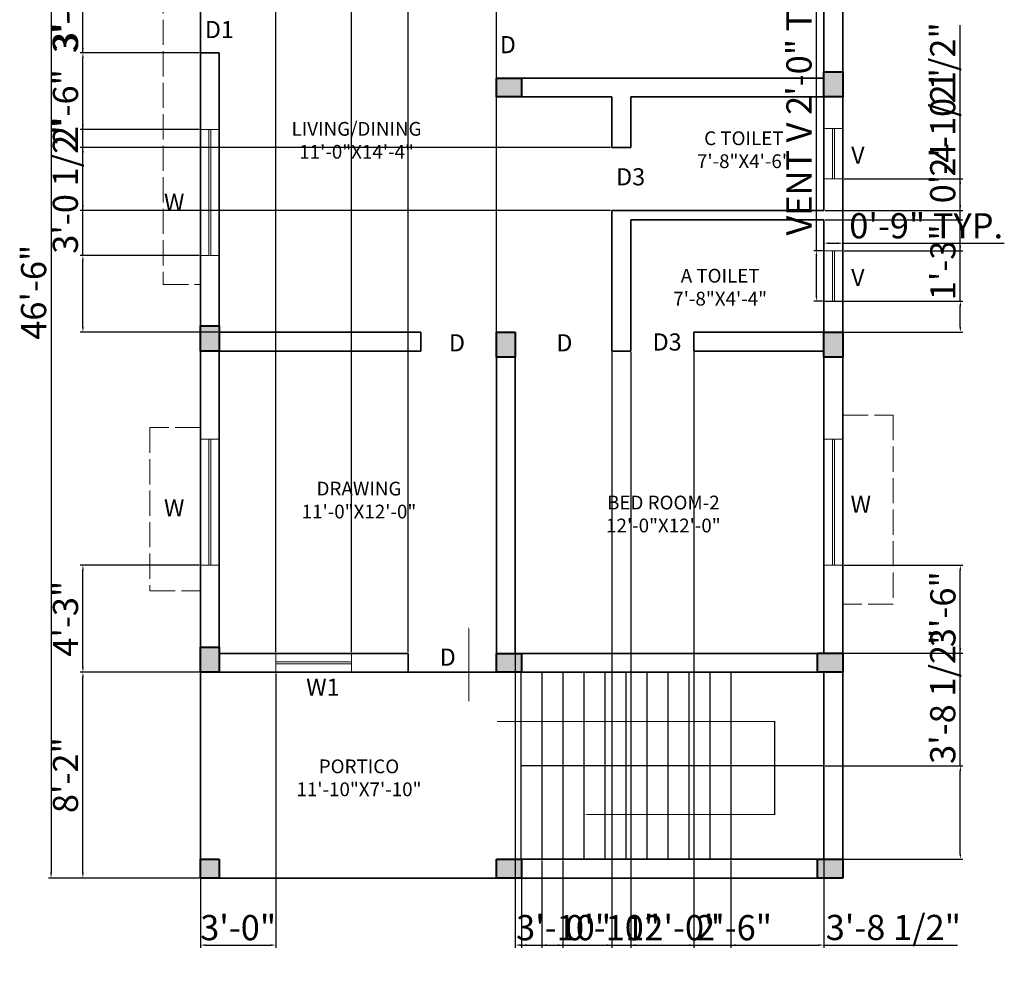
# Model space of a CAD drawing. Units: inches. Extents: x 27449 to 27965, y 46348 to 47103.
# Tile 1 of 2: x 27449 to 27918, y 46348 to 46800. Entities that reach past the tile are written whole.
import ezdxf

# ---------------------------------------------------------------- set-up
doc = ezdxf.new("R2010")
doc.units = ezdxf.units.IN
doc.linetypes.add('ACAD_ISO02W100', pattern=[15, 12, -3])
for name, color, linetype, lineweight in [('A-ANNO-DIMS', 2, 'Continuous', 18), ('A-ANNO-SYMB', 7, 'Continuous', 18), ('A-ANNO-TEXT', 7, 'Continuous', 18), ('A-AREA-IDEN', 7, 'Continuous', 20), ('A-COLS', 7, 'Continuous', 40), ('A-COLS-PATT', 252, 'Continuous', 13), ('A-FLOR-STRS', 7, 'Continuous', 25), ('A-GLAZ', 4, 'Continuous', 20), ('A-GLAZ-OVHD', 8, 'ACAD_ISO02W100', 13), ('A-WALL', 7, 'Continuous', 35)]:
    doc.layers.add(name, color=color, linetype=linetype, lineweight=lineweight)
doc.styles.get("Standard").update_dxf_attribs({"font": 'arial.ttf'})
doc.dimstyles.new('ISO-25', dxfattribs={"dimtxt": 12, "dimasz": 2.5, "dimexe": 1.25, "dimexo": 0.625, "dimtad": 1, "dimlunit": 3, "dimtxsty": 'Standard', "dimcen": 2.5, "dimadec": 0, "dimazin": 0, "dimtfac": 1, "dimtmove": 0, "dimatfit": 3, "dimfxl": 1, "dimarcsym": 0})

# ---------------------------------------------------------------- blocks, each defined once
blk = doc.blocks.new('*D1')
at = {"layer": 'A-ANNO-DIMS', "color": 0, "lineweight": -2, "transparency": 16777216}
for p, q in [((27534.79, 46948.86), (27463.05, 46948.86)), ((27464.3, 46946.36), (27464.3, 46393.36)), ((27534.79, 46390.86), (27463.05, 46390.86))]:
    blk.add_line(p, q, dxfattribs=at)
at = {"layer": 'A-ANNO-DIMS', "color": 0, "transparency": 16777216}
for points in [[(27463.88, 46946.36), (27464.71, 46946.36), (27464.3, 46948.86)], [(27463.88, 46393.36), (27464.71, 46393.36), (27464.3, 46390.86)]]:
    blk.add_solid(points, dxfattribs=at)
at = {"layer": 'Defpoints', "color": 0, "transparency": 16777216}
for p in [(27535.42, 46948.86), (27464.3, 46390.86), (27535.42, 46390.86)]:
    blk.add_point(p, dxfattribs=at)
at = {"layer": 'A-ANNO-DIMS', "color": 0, "transparency": 16777216, "insert": (27457.54, 46669.86), "char_height": 12, "attachment_point": 5, "rotation": 90}
blk.add_mtext('46\'-6"', dxfattribs=at)
blk = doc.blocks.new('WIN-W-60IN')
for p, q in [((0, 60), (9, 60)), ((0, 0), (0, 60)), ((4, 0), (4, 60)), ((5, 0), (5, 60)), ((9, 60), (9, 0)), ((9, 0), (0, 0))]:
    blk.add_line(p, q)
blk = doc.blocks.new('VENT-V-24IN')
for p, q in [((0, 0), (0, 24)), ((0, 24), (9, 24)), ((4, 24), (4, 0)), ((5, 24), (5, 0)), ((9, 24), (9, 0)), ((0, 0), (9, 0))]:
    blk.add_line(p, q)
blk = doc.blocks.new('COL-9X12IN')
h = blk.add_hatch(color=256)
h.dxf.hatch_style = 1
h.paths.add_polyline_path([(9, 12), (0, 12), (0, 0), (9, 0)])
for p, q in [((0, 12), (9, 12)), ((0, 0), (0, 12)), ((9, 12), (9, 0)), ((9, 0), (0, 0))]:
    blk.add_line(p, q)
blk = doc.blocks.new('ENTRY-ARROW')
blk.add_lwpolyline([(0, 0, 0.5, 0.5, 0), (0, 22.23, 5, 0, 0), (0, 35.55, 0, 0, 0)], format="xyseb")
blk = doc.blocks.new('*D11')
at = {"layer": 'A-ANNO-DIMS', "color": 0, "lineweight": -2, "transparency": 16777216}
for p, q in [((27828.82, 46689.61), (27828.82, 46832.34)), ((27831.79, 46689.61), (27827.57, 46689.61)), ((27828.82, 46668.11), (27828.82, 46687.11)), ((27831.79, 46665.61), (27827.57, 46665.61))]:
    blk.add_line(p, q, dxfattribs=at)
at = {"layer": 'A-ANNO-DIMS', "color": 0, "transparency": 16777216}
for points in [[(27828.4, 46687.11), (27829.24, 46687.11), (27828.82, 46689.61)], [(27828.4, 46668.11), (27829.24, 46668.11), (27828.82, 46665.61)]]:
    blk.add_solid(points, dxfattribs=at)
at = {"layer": 'Defpoints', "color": 0, "transparency": 16777216}
for p in [(27828.82, 46689.61), (27832.42, 46689.61), (27832.42, 46665.61)]:
    blk.add_point(p, dxfattribs=at)
at = {"layer": 'A-ANNO-DIMS', "color": 0, "transparency": 16777216, "insert": (27822.07, 46762.22), "char_height": 12, "attachment_point": 5, "rotation": 90}
blk.add_mtext('VENT V 2\'-0" TYP.', dxfattribs=at)
blk = doc.blocks.new('*D12')
at = {"layer": 'A-ANNO-DIMS', "color": 0, "lineweight": -2, "transparency": 16777216}
for p, q in [((27832.42, 46690.24), (27832.42, 46694.46)), ((27841.42, 46690.24), (27841.42, 46694.46)), ((27834.92, 46693.21), (27838.92, 46693.21)), ((27841.42, 46693.21), (27918.32, 46693.21))]:
    blk.add_line(p, q, dxfattribs=at)
at = {"layer": 'A-ANNO-DIMS', "color": 0, "transparency": 16777216}
for points in [[(27834.92, 46693.63), (27834.92, 46692.8), (27832.42, 46693.21)], [(27838.92, 46693.63), (27838.92, 46692.8), (27841.42, 46693.21)]]:
    blk.add_solid(points, dxfattribs=at)
at = {"layer": 'Defpoints', "color": 0, "transparency": 16777216}
for p in [(27832.42, 46689.61), (27841.42, 46693.21), (27841.42, 46689.61)]:
    blk.add_point(p, dxfattribs=at)
at = {"layer": 'A-ANNO-DIMS', "color": 0, "transparency": 16777216, "insert": (27881.12, 46699.96), "char_height": 12, "attachment_point": 5}
blk.add_mtext('0\'-9" TYP.', dxfattribs=at)
blk = doc.blocks.new('*D13')
at = {"layer": 'A-ANNO-DIMS', "color": 0, "lineweight": -2, "transparency": 16777216}
for p, q in [((27534.79, 46488.86), (27478.22, 46488.86)), ((27479.47, 46393.36), (27479.47, 46486.36)), ((27534.79, 46390.86), (27478.22, 46390.86))]:
    blk.add_line(p, q, dxfattribs=at)
at = {"layer": 'A-ANNO-DIMS', "color": 0, "transparency": 16777216}
for points in [[(27479.05, 46486.36), (27479.89, 46486.36), (27479.47, 46488.86)], [(27479.05, 46393.36), (27479.89, 46393.36), (27479.47, 46390.86)]]:
    blk.add_solid(points, dxfattribs=at)
at = {"layer": 'Defpoints', "color": 0, "transparency": 16777216}
for p in [(27479.47, 46488.86), (27535.42, 46488.86), (27535.42, 46390.86)]:
    blk.add_point(p, dxfattribs=at)
at = {"layer": 'A-ANNO-DIMS', "color": 0, "transparency": 16777216, "insert": (27472.72, 46439.86), "char_height": 12, "attachment_point": 5, "rotation": 90}
blk.add_mtext('8\'-2"', dxfattribs=at)
blk = doc.blocks.new('*D14')
at = {"layer": 'A-ANNO-DIMS', "color": 0, "lineweight": -2, "transparency": 16777216}
for p, q in [((27534.79, 46539.86), (27478.22, 46539.86)), ((27479.47, 46491.36), (27479.47, 46537.36)), ((27534.79, 46488.86), (27478.22, 46488.86))]:
    blk.add_line(p, q, dxfattribs=at)
at = {"layer": 'A-ANNO-DIMS', "color": 0, "transparency": 16777216}
for points in [[(27479.05, 46537.36), (27479.89, 46537.36), (27479.47, 46539.86)], [(27479.05, 46491.36), (27479.89, 46491.36), (27479.47, 46488.86)]]:
    blk.add_solid(points, dxfattribs=at)
at = {"layer": 'Defpoints', "color": 0, "transparency": 16777216}
for p in [(27479.47, 46539.86), (27535.42, 46539.86), (27535.42, 46488.86)]:
    blk.add_point(p, dxfattribs=at)
at = {"layer": 'A-ANNO-DIMS', "color": 0, "transparency": 16777216, "insert": (27472.71, 46514.36), "char_height": 12, "attachment_point": 5, "rotation": 90}
blk.add_mtext('4\'-3"', dxfattribs=at)
blk = doc.blocks.new('*D15')
at = {"layer": 'A-ANNO-DIMS', "color": 0, "lineweight": -2, "transparency": 16777216}
for p, q in [((27479.47, 46687.36), (27479.47, 46750.97)), ((27534.79, 46687.36), (27478.22, 46687.36)), ((27479.47, 46653.36), (27479.47, 46684.86)), ((27543.79, 46650.86), (27478.22, 46650.86))]:
    blk.add_line(p, q, dxfattribs=at)
at = {"layer": 'A-ANNO-DIMS', "color": 0, "transparency": 16777216}
for points in [[(27479.05, 46684.86), (27479.89, 46684.86), (27479.47, 46687.36)], [(27479.05, 46653.36), (27479.89, 46653.36), (27479.47, 46650.86)]]:
    blk.add_solid(points, dxfattribs=at)
at = {"layer": 'Defpoints', "color": 0, "transparency": 16777216}
for p in [(27479.47, 46687.36), (27535.42, 46687.36), (27544.42, 46650.86)]:
    blk.add_point(p, dxfattribs=at)
at = {"layer": 'A-ANNO-DIMS', "color": 0, "transparency": 16777216, "insert": (27472.64, 46720.41), "char_height": 12, "attachment_point": 5, "rotation": 90}
blk.add_mtext('3\'-0 1/2"', dxfattribs=at)
blk = doc.blocks.new('*D16')
at = {"layer": 'A-ANNO-DIMS', "color": 0, "lineweight": -2, "transparency": 16777216}
for p, q in [((27479.47, 46783.86), (27479.47, 46847.47)), ((27534.79, 46783.86), (27478.22, 46783.86)), ((27479.47, 46749.86), (27479.47, 46781.36)), ((27534.79, 46747.36), (27478.22, 46747.36))]:
    blk.add_line(p, q, dxfattribs=at)
at = {"layer": 'A-ANNO-DIMS', "color": 0, "transparency": 16777216}
for points in [[(27479.05, 46781.36), (27479.89, 46781.36), (27479.47, 46783.86)], [(27479.05, 46749.86), (27479.89, 46749.86), (27479.47, 46747.36)]]:
    blk.add_solid(points, dxfattribs=at)
at = {"layer": 'Defpoints', "color": 0, "transparency": 16777216}
for p in [(27479.47, 46783.86), (27535.42, 46783.86), (27535.42, 46747.36)]:
    blk.add_point(p, dxfattribs=at)
at = {"layer": 'A-ANNO-DIMS', "color": 0, "transparency": 16777216, "insert": (27472.64, 46816.91), "char_height": 12, "attachment_point": 5, "rotation": 90}
blk.add_mtext('3\'-0 1/2"', dxfattribs=at)
blk = doc.blocks.new('*D17')
at = {"layer": 'A-ANNO-DIMS', "color": 0, "lineweight": -2, "transparency": 16777216}
for p, q in [((27534.79, 46819.86), (27478.22, 46819.86)), ((27479.47, 46786.36), (27479.47, 46817.36)), ((27534.79, 46783.86), (27478.22, 46783.86))]:
    blk.add_line(p, q, dxfattribs=at)
at = {"layer": 'A-ANNO-DIMS', "color": 0, "transparency": 16777216}
for points in [[(27479.05, 46817.36), (27479.89, 46817.36), (27479.47, 46819.86)], [(27479.05, 46786.36), (27479.89, 46786.36), (27479.47, 46783.86)]]:
    blk.add_solid(points, dxfattribs=at)
at = {"layer": 'Defpoints', "color": 0, "transparency": 16777216}
for p in [(27479.47, 46819.86), (27535.42, 46819.86), (27535.42, 46783.86)]:
    blk.add_point(p, dxfattribs=at)
at = {"layer": 'A-ANNO-DIMS', "color": 0, "transparency": 16777216, "insert": (27472.71, 46801.86), "char_height": 12, "attachment_point": 5, "rotation": 90}
blk.add_mtext('3\'-0"', dxfattribs=at)
blk = doc.blocks.new('*D20')
at = {"layer": 'A-ANNO-DIMS', "color": 0, "lineweight": -2, "transparency": 16777216}
for p, q in [((27571.42, 46498.49), (27571.42, 47006.06)), ((27573.92, 47004.81), (27604.92, 47004.81)), ((27607.42, 46498.49), (27607.42, 47006.06))]:
    blk.add_line(p, q, dxfattribs=at)
at = {"layer": 'A-ANNO-DIMS', "color": 0, "transparency": 16777216}
for points in [[(27573.92, 47005.23), (27573.92, 47004.4), (27571.42, 47004.81)], [(27604.92, 47005.23), (27604.92, 47004.4), (27607.42, 47004.81)]]:
    blk.add_solid(points, dxfattribs=at)
at = {"layer": 'Defpoints', "color": 0, "transparency": 16777216}
for p in [(27607.42, 47004.81), (27571.42, 46497.86), (27607.42, 46497.86)]:
    blk.add_point(p, dxfattribs=at)
at = {"layer": 'A-ANNO-DIMS', "color": 0, "transparency": 16777216, "insert": (27589.42, 47011.57), "char_height": 12, "attachment_point": 5}
blk.add_mtext('3\'-0"', dxfattribs=at)
blk = doc.blocks.new('*D21')
at = {"layer": 'A-ANNO-DIMS', "color": 0, "lineweight": -2, "transparency": 16777216}
for p, q in [((27535.42, 46488.24), (27535.42, 46357.66)), ((27571.42, 46488.24), (27571.42, 46357.66)), ((27537.92, 46358.91), (27568.92, 46358.91))]:
    blk.add_line(p, q, dxfattribs=at)
at = {"layer": 'A-ANNO-DIMS', "color": 0, "transparency": 16777216}
for points in [[(27537.92, 46359.33), (27537.92, 46358.5), (27535.42, 46358.91)], [(27568.92, 46359.33), (27568.92, 46358.5), (27571.42, 46358.91)]]:
    blk.add_solid(points, dxfattribs=at)
at = {"layer": 'Defpoints', "color": 0, "transparency": 16777216}
for p in [(27535.42, 46488.86), (27571.42, 46488.86), (27571.42, 46358.91)]:
    blk.add_point(p, dxfattribs=at)
at = {"layer": 'A-ANNO-DIMS', "color": 0, "transparency": 16777216, "insert": (27553.42, 46365.67), "char_height": 12, "attachment_point": 5}
blk.add_mtext('3\'-0"', dxfattribs=at)
blk = doc.blocks.new('*D22')
at = {"layer": 'A-ANNO-DIMS', "color": 0, "lineweight": -2, "transparency": 16777216}
for p, q in [((27634.42, 46498.49), (27634.42, 47006.06)), ((27636.92, 47004.81), (27673.92, 47004.81)), ((27676.42, 46498.49), (27676.42, 47006.06))]:
    blk.add_line(p, q, dxfattribs=at)
at = {"layer": 'A-ANNO-DIMS', "color": 0, "transparency": 16777216}
for points in [[(27636.92, 47005.23), (27636.92, 47004.4), (27634.42, 47004.81)], [(27673.92, 47005.23), (27673.92, 47004.4), (27676.42, 47004.81)]]:
    blk.add_solid(points, dxfattribs=at)
at = {"layer": 'Defpoints', "color": 0, "transparency": 16777216}
for p in [(27676.42, 47004.81), (27634.42, 46497.86), (27676.42, 46497.86)]:
    blk.add_point(p, dxfattribs=at)
at = {"layer": 'A-ANNO-DIMS', "color": 0, "transparency": 16777216, "insert": (27655.42, 47011.57), "char_height": 12, "attachment_point": 5}
blk.add_mtext('3\'-6"', dxfattribs=at)
blk = doc.blocks.new('*D23')
at = {"layer": 'A-ANNO-DIMS', "color": 0, "lineweight": -2, "transparency": 16777216}
for p, q in [((27688.42, 46399.24), (27688.42, 46357.66)), ((27832.42, 46399.24), (27832.42, 46357.66)), ((27690.92, 46358.91), (27829.92, 46358.91))]:
    blk.add_line(p, q, dxfattribs=at)
at = {"layer": 'A-ANNO-DIMS', "color": 0, "transparency": 16777216}
for points in [[(27690.92, 46359.33), (27690.92, 46358.5), (27688.42, 46358.91)], [(27829.92, 46359.33), (27829.92, 46358.5), (27832.42, 46358.91)]]:
    blk.add_solid(points, dxfattribs=at)
at = {"layer": 'Defpoints', "color": 0, "transparency": 16777216}
for p in [(27688.42, 46399.86), (27832.42, 46399.86), (27832.42, 46358.91)]:
    blk.add_point(p, dxfattribs=at)
at = {"layer": 'A-ANNO-DIMS', "color": 0, "transparency": 16777216, "insert": (27760.42, 46365.66), "char_height": 12, "attachment_point": 5}
blk.add_mtext('12\'-0"', dxfattribs=at)
blk = doc.blocks.new('*D24')
at = {"layer": 'A-ANNO-DIMS', "color": 0, "lineweight": -2, "transparency": 16777216}
for p, q in [((27788.02, 46399.24), (27788.02, 46357.66)), ((27832.42, 46399.24), (27832.42, 46357.66)), ((27790.52, 46358.91), (27829.92, 46358.91)), ((27832.42, 46358.91), (27896.02, 46358.91))]:
    blk.add_line(p, q, dxfattribs=at)
at = {"layer": 'A-ANNO-DIMS', "color": 0, "transparency": 16777216}
for points in [[(27790.52, 46359.33), (27790.52, 46358.5), (27788.02, 46358.91)], [(27829.92, 46359.33), (27829.92, 46358.5), (27832.42, 46358.91)]]:
    blk.add_solid(points, dxfattribs=at)
at = {"layer": 'Defpoints', "color": 0, "transparency": 16777216}
for p in [(27788.02, 46399.86), (27832.42, 46399.86), (27832.42, 46358.91)]:
    blk.add_point(p, dxfattribs=at)
at = {"layer": 'A-ANNO-DIMS', "color": 0, "transparency": 16777216, "insert": (27865.47, 46365.75), "char_height": 12, "attachment_point": 5}
blk.add_mtext('3\'-8 1/2"', dxfattribs=at)
blk = doc.blocks.new('*D25')
at = {"layer": 'A-ANNO-DIMS', "color": 0, "lineweight": -2, "transparency": 16777216}
for p, q in [((27698.02, 46399.24), (27698.02, 46357.66)), ((27708.02, 46399.24), (27708.02, 46357.66)), ((27700.52, 46358.91), (27705.52, 46358.91)), ((27708.02, 46358.91), (27752.99, 46358.91))]:
    blk.add_line(p, q, dxfattribs=at)
at = {"layer": 'A-ANNO-DIMS', "color": 0, "transparency": 16777216}
for points in [[(27700.52, 46359.33), (27700.52, 46358.5), (27698.02, 46358.91)], [(27705.52, 46359.33), (27705.52, 46358.5), (27708.02, 46358.91)]]:
    blk.add_solid(points, dxfattribs=at)
at = {"layer": 'Defpoints', "color": 0, "transparency": 16777216}
for p in [(27698.02, 46399.86), (27708.02, 46399.86), (27708.02, 46358.91)]:
    blk.add_point(p, dxfattribs=at)
at = {"layer": 'A-ANNO-DIMS', "color": 0, "transparency": 16777216, "insert": (27731.76, 46365.66), "char_height": 12, "attachment_point": 5}
blk.add_mtext('0\'-10"', dxfattribs=at)
blk = doc.blocks.new('*D26')
at = {"layer": 'A-ANNO-DIMS', "color": 0, "lineweight": -2, "transparency": 16777216}
for p, q in [((27897.37, 46444.36), (27897.37, 46507.97)), ((27833.04, 46444.36), (27898.62, 46444.36)), ((27897.37, 46402.36), (27897.37, 46441.86)), ((27833.04, 46399.86), (27898.62, 46399.86))]:
    blk.add_line(p, q, dxfattribs=at)
at = {"layer": 'A-ANNO-DIMS', "color": 0, "transparency": 16777216}
for points in [[(27896.95, 46441.86), (27897.79, 46441.86), (27897.37, 46444.36)], [(27896.95, 46402.36), (27897.79, 46402.36), (27897.37, 46399.86)]]:
    blk.add_solid(points, dxfattribs=at)
at = {"layer": 'Defpoints', "color": 0, "transparency": 16777216}
for p in [(27832.42, 46444.36), (27897.37, 46444.36), (27832.42, 46399.86)]:
    blk.add_point(p, dxfattribs=at)
at = {"layer": 'A-ANNO-DIMS', "color": 0, "transparency": 16777216, "insert": (27890.54, 46477.41), "char_height": 12, "attachment_point": 5, "rotation": 90}
blk.add_mtext('3\'-8 1/2"', dxfattribs=at)
blk = doc.blocks.new('*D29')
at = {"layer": 'A-ANNO-DIMS', "color": 0, "lineweight": -2, "transparency": 16777216}
for p, q in [((27842.04, 46539.86), (27898.62, 46539.86)), ((27897.37, 46500.39), (27897.37, 46537.36)), ((27842.04, 46497.89), (27898.62, 46497.89))]:
    blk.add_line(p, q, dxfattribs=at)
at = {"layer": 'A-ANNO-DIMS', "color": 0, "transparency": 16777216}
for points in [[(27896.95, 46537.36), (27897.79, 46537.36), (27897.37, 46539.86)], [(27896.95, 46500.39), (27897.79, 46500.39), (27897.37, 46497.89)]]:
    blk.add_solid(points, dxfattribs=at)
at = {"layer": 'Defpoints', "color": 0, "transparency": 16777216}
for p in [(27841.42, 46539.86), (27897.37, 46539.86), (27841.42, 46497.89)]:
    blk.add_point(p, dxfattribs=at)
at = {"layer": 'A-ANNO-DIMS', "color": 0, "transparency": 16777216, "insert": (27890.61, 46518.87), "char_height": 12, "attachment_point": 5, "rotation": 90}
blk.add_mtext('3\'-6"', dxfattribs=at)
blk = doc.blocks.new('*D30')
at = {"layer": 'A-ANNO-DIMS', "color": 0, "lineweight": -2, "transparency": 16777216}
for p, q in [((27897.37, 46723.86), (27897.37, 46797)), ((27842.04, 46723.86), (27898.62, 46723.86)), ((27897.37, 46692.11), (27897.37, 46721.36)), ((27842.04, 46689.61), (27898.62, 46689.61))]:
    blk.add_line(p, q, dxfattribs=at)
at = {"layer": 'A-ANNO-DIMS', "color": 0, "transparency": 16777216}
for points in [[(27896.95, 46721.36), (27897.79, 46721.36), (27897.37, 46723.86)], [(27896.95, 46692.11), (27897.79, 46692.11), (27897.37, 46689.61)]]:
    blk.add_solid(points, dxfattribs=at)
at = {"layer": 'Defpoints', "color": 0, "transparency": 16777216}
for p in [(27841.42, 46723.86), (27897.37, 46723.86), (27841.42, 46689.61)]:
    blk.add_point(p, dxfattribs=at)
at = {"layer": 'A-ANNO-DIMS', "color": 0, "transparency": 16777216, "insert": (27890.54, 46761.68), "char_height": 12, "attachment_point": 5, "rotation": 90}
blk.add_mtext('2\'-10 1/2"', dxfattribs=at)
blk = doc.blocks.new('*D31')
at = {"layer": 'A-ANNO-DIMS', "color": 0, "lineweight": -2, "transparency": 16777216}
for p, q in [((27897.37, 46665.61), (27897.37, 46700.13)), ((27833.04, 46665.61), (27898.62, 46665.61)), ((27897.37, 46653.36), (27897.37, 46663.11)), ((27833.04, 46650.86), (27898.62, 46650.86))]:
    blk.add_line(p, q, dxfattribs=at)
at = {"layer": 'A-ANNO-DIMS', "color": 0, "transparency": 16777216}
for points in [[(27896.95, 46663.11), (27897.79, 46663.11), (27897.37, 46665.61)], [(27896.95, 46653.36), (27897.79, 46653.36), (27897.37, 46650.86)]]:
    blk.add_solid(points, dxfattribs=at)
at = {"layer": 'Defpoints', "color": 0, "transparency": 16777216}
for p in [(27832.42, 46665.61), (27897.37, 46665.61), (27832.42, 46650.86)]:
    blk.add_point(p, dxfattribs=at)
at = {"layer": 'A-ANNO-DIMS', "color": 0, "transparency": 16777216, "insert": (27890.61, 46684.12), "char_height": 12, "attachment_point": 5, "rotation": 90}
blk.add_mtext('1\'-3"', dxfattribs=at)
blk = doc.blocks.new('*D32')
at = {"layer": 'A-ANNO-DIMS', "color": 0, "lineweight": -2, "transparency": 16777216}
for p, q in [((27740.42, 46641.24), (27740.42, 46357.66)), ((27770.42, 46641.24), (27770.42, 46357.66)), ((27742.92, 46358.91), (27767.92, 46358.91)), ((27770.42, 46358.91), (27806.27, 46358.91))]:
    blk.add_line(p, q, dxfattribs=at)
at = {"layer": 'A-ANNO-DIMS', "color": 0, "transparency": 16777216}
for points in [[(27742.92, 46359.33), (27742.92, 46358.5), (27740.42, 46358.91)], [(27767.92, 46359.33), (27767.92, 46358.5), (27770.42, 46358.91)]]:
    blk.add_solid(points, dxfattribs=at)
at = {"layer": 'Defpoints', "color": 0, "transparency": 16777216}
for p in [(27740.42, 46641.86), (27770.42, 46641.86), (27770.42, 46358.91)]:
    blk.add_point(p, dxfattribs=at)
at = {"layer": 'A-ANNO-DIMS', "color": 0, "transparency": 16777216, "insert": (27789.6, 46365.66), "char_height": 12, "attachment_point": 5}
blk.add_mtext('2\'-6"', dxfattribs=at)
blk = doc.blocks.new('*D33')
at = {"layer": 'A-ANNO-DIMS', "color": 0, "lineweight": -2, "transparency": 16777216}
for p, q in [((27685.42, 46638.24), (27685.42, 46357.66)), ((27731.42, 46641.24), (27731.42, 46357.66)), ((27687.92, 46358.91), (27728.92, 46358.91))]:
    blk.add_line(p, q, dxfattribs=at)
at = {"layer": 'A-ANNO-DIMS', "color": 0, "transparency": 16777216}
for points in [[(27687.92, 46359.33), (27687.92, 46358.5), (27685.42, 46358.91)], [(27728.92, 46359.33), (27728.92, 46358.5), (27731.42, 46358.91)]]:
    blk.add_solid(points, dxfattribs=at)
at = {"layer": 'Defpoints', "color": 0, "transparency": 16777216}
for p in [(27731.42, 46641.86), (27685.42, 46638.86), (27731.42, 46358.91)]:
    blk.add_point(p, dxfattribs=at)
at = {"layer": 'A-ANNO-DIMS', "color": 0, "transparency": 16777216, "insert": (27708.42, 46365.67), "char_height": 12, "attachment_point": 5}
blk.add_mtext('3\'-10"', dxfattribs=at)
blk = doc.blocks.new('*D34')
at = {"layer": 'A-ANNO-DIMS', "color": 0, "lineweight": -2, "transparency": 16777216}
for p, q in [((27479.47, 46738.86), (27479.47, 46774.72)), ((27730.79, 46738.86), (27478.22, 46738.86)), ((27479.47, 46711.36), (27479.47, 46736.36)), ((27730.79, 46708.86), (27478.22, 46708.86))]:
    blk.add_line(p, q, dxfattribs=at)
at = {"layer": 'A-ANNO-DIMS', "color": 0, "transparency": 16777216}
for points in [[(27479.05, 46736.36), (27479.89, 46736.36), (27479.47, 46738.86)], [(27479.05, 46711.36), (27479.89, 46711.36), (27479.47, 46708.86)]]:
    blk.add_solid(points, dxfattribs=at)
at = {"layer": 'Defpoints', "color": 0, "transparency": 16777216}
for p in [(27479.47, 46738.86), (27731.42, 46738.86), (27731.42, 46708.86)]:
    blk.add_point(p, dxfattribs=at)
at = {"layer": 'A-ANNO-DIMS', "color": 0, "transparency": 16777216, "insert": (27472.72, 46758.04), "char_height": 12, "attachment_point": 5, "rotation": 90}
blk.add_mtext('2\'-6"', dxfattribs=at)
blk = doc.blocks.new('*D35')
at = {"layer": 'A-ANNO-DIMS', "color": 0, "lineweight": -2, "transparency": 16777216}
for p, q in [((27897.37, 46711.36), (27897.37, 46774.97)), ((27833.04, 46708.86), (27898.62, 46708.86)), ((27897.37, 46704.36), (27897.37, 46708.86)), ((27833.04, 46704.36), (27898.62, 46704.36)), ((27897.37, 46701.86), (27897.37, 46699.36))]:
    blk.add_line(p, q, dxfattribs=at)
at = {"layer": 'A-ANNO-DIMS', "color": 0, "transparency": 16777216}
for points in [[(27896.95, 46711.36), (27897.79, 46711.36), (27897.37, 46708.86)], [(27896.95, 46701.86), (27897.79, 46701.86), (27897.37, 46704.36)]]:
    blk.add_solid(points, dxfattribs=at)
at = {"layer": 'Defpoints', "color": 0, "transparency": 16777216}
for p in [(27832.42, 46708.86), (27897.37, 46708.86), (27832.42, 46704.36)]:
    blk.add_point(p, dxfattribs=at)
at = {"layer": 'A-ANNO-DIMS', "color": 0, "transparency": 16777216, "insert": (27890.54, 46744.42), "char_height": 12, "attachment_point": 5, "rotation": 90}
blk.add_mtext('0\'-4 1/2"', dxfattribs=at)

msp = doc.modelspace()

# ---------------------------------------------------------------- hatches: boundary and pattern name
at = {"layer": 'A-COLS-PATT'}
h = msp.add_hatch(color=256, dxfattribs=at)
h.dxf.hatch_style = 1
h.paths.add_polyline_path([(27544.42, 46399.862), (27535.42, 46399.862), (27535.42, 46390.862), (27544.42, 46390.862)])

# ---------------------------------------------------------------- linework, layer by layer
at = {"layer": 'A-COLS'}
for p, q in [((27535.42, 46399.862), (27544.42, 46399.862)), ((27535.42, 46390.862), (27535.42, 46399.862)), ((27544.42, 46399.862), (27544.42, 46390.862)), ((27544.42, 46390.862), (27535.42, 46390.862))]:
    msp.add_line(p, q, dxfattribs=at)
at = {"layer": 'A-FLOR-STRS'}
for p, q in [((27688.02, 46488.862), (27688.02, 46399.862)), ((27698.02, 46488.862), (27698.02, 46399.862)), ((27708.02, 46488.862), (27708.02, 46399.862)), ((27718.02, 46488.862), (27718.02, 46399.862)), ((27728.02, 46488.862), (27728.02, 46399.862)), ((27738.02, 46488.862), (27738.02, 46399.862)), ((27748.02, 46488.862), (27748.02, 46399.862)), ((27758.02, 46488.862), (27758.02, 46399.862)), ((27768.02, 46488.862), (27768.02, 46399.862)), ((27778.02, 46488.862), (27778.02, 46399.862)), ((27788.02, 46488.862), (27788.02, 46399.862)), ((27832.42, 46444.362), (27688.02, 46444.362))]:
    msp.add_line(p, q, dxfattribs=at)
msp.add_lwpolyline([(27676.661, 46465.348, 0.5, 0.5, 0), (27748.02, 46465.348, 2, 0.5, 0), (27753.233, 46465.348, 0.5, 0.5, 0), (27808.951, 46465.348, 0.5, 0.5, 0), (27808.951, 46449.602, 2, 0, 0), (27808.951, 46444.362, 0.5, 0.5, 0), (27808.951, 46421.116, 0.5, 0.5, 0), (27738.02, 46421.116, 5, 0, 0), (27718.02, 46421.116, 0, 0, 0)], format="xyseb", dxfattribs=at)
at = {"layer": 'A-GLAZ'}
for p, q in [((27571.42, 46488.862), (27571.42, 46497.862)), ((27571.42, 46497.862), (27607.42, 46497.862)), ((27607.42, 46488.862), (27607.42, 46497.862)), ((27571.42, 46493.862), (27607.42, 46493.862)), ((27571.42, 46492.862), (27607.42, 46492.862)), ((27607.42, 46488.862), (27571.42, 46488.862))]:
    msp.add_line(p, q, dxfattribs=at)
at = {"layer": 'A-GLAZ-OVHD'}
for p, q in [((27517.698, 46919.634), (27517.698, 46673.583)), ((27517.698, 46673.583), (27535.42, 46673.583)), ((27841.42, 46611.349), (27865.42, 46611.349)), ((27865.42, 46611.349), (27865.42, 46521.298)), ((27535.42, 46605.362), (27511.42, 46605.362)), ((27511.42, 46605.362), (27511.42, 46527.625)), ((27511.42, 46527.625), (27535.42, 46527.625)), ((27865.42, 46521.298), (27841.42, 46521.298))]:
    msp.add_line(p, q, dxfattribs=at)
at = {"layer": 'A-WALL'}
for p, q in [((27841.42, 46948.862), (27841.42, 46390.862)), ((27832.42, 46939.862), (27832.42, 46771.862)), ((27535.42, 46390.862), (27535.42, 46819.862)), ((27544.42, 46783.862), (27535.42, 46783.862)), ((27544.42, 46650.862), (27544.42, 46783.862)), ((27676.42, 46762.862), (27676.42, 46771.862)), ((27685.42, 46771.862), (27676.42, 46771.862)), ((27685.42, 46771.862), (27832.42, 46771.862)), ((27676.42, 46762.862), (27731.42, 46762.862)), ((27731.42, 46762.862), (27731.42, 46738.862)), ((27740.42, 46762.862), (27740.42, 46738.862)), ((27740.42, 46762.862), (27832.42, 46762.862)), ((27832.42, 46762.862), (27832.42, 46708.862)), ((27731.42, 46738.862), (27740.42, 46738.862)), ((27731.42, 46708.862), (27832.42, 46708.862)), ((27731.42, 46708.862), (27731.42, 46641.862)), ((27740.42, 46704.362), (27832.42, 46704.362)), ((27740.42, 46704.362), (27740.42, 46641.862)), ((27832.42, 46704.362), (27832.42, 46650.862)), ((27544.42, 46650.862), (27640.42, 46650.862)), ((27640.42, 46641.862), (27640.42, 46650.862)), ((27676.42, 46497.862), (27676.42, 46650.862)), ((27676.42, 46650.862), (27685.42, 46650.862)), ((27685.42, 46497.862), (27685.42, 46650.862)), ((27770.42, 46650.862), (27770.42, 46641.862)), ((27770.42, 46650.862), (27832.42, 46650.862)), ((27544.42, 46641.862), (27640.42, 46641.862)), ((27544.42, 46497.862), (27544.42, 46641.862)), ((27731.42, 46641.862), (27740.42, 46641.862)), ((27770.42, 46641.862), (27832.42, 46641.862)), ((27832.42, 46641.862), (27832.42, 46497.862)), ((27544.42, 46497.862), (27634.42, 46497.862)), ((27634.42, 46497.862), (27634.42, 46488.862)), ((27676.42, 46497.862), (27676.42, 46488.862)), ((27685.42, 46497.862), (27832.42, 46497.862)), ((27535.42, 46488.862), (27676.42, 46488.862)), ((27676.42, 46488.862), (27832.42, 46488.862)), ((27832.42, 46488.862), (27832.42, 46399.862)), ((27832.42, 46399.862), (27676.42, 46399.862)), ((27841.42, 46390.862), (27535.42, 46390.862))]:
    msp.add_line(p, q, dxfattribs=at)

# ---------------------------------------------------------------- block references
at = {"layer": 'A-ANNO-SYMB'}
msp.add_blockref('ENTRY-ARROW', (27663.231, 46474.957), dxfattribs=at)
at = {"layer": 'A-COLS'}
for p in [(27832.42, 46762.862), (27535.42, 46641.862), (27676.42, 46638.862), (27832.42, 46638.862), (27535.42, 46488.862)]:
    msp.add_blockref('COL-9X12IN', p, dxfattribs=at)
for p, rotation in [((27688.42, 46762.862), 90.00000000005677), ((27688.42, 46488.862), 90.00000000001548), ((27841.42, 46488.885), 90.00000000001548), ((27688.42, 46390.862), 90.00000000005677), ((27841.42, 46390.862), 90.00000000005677)]:
    msp.add_blockref('COL-9X12IN', p, dxfattribs=dict(at, rotation=rotation))
at = {"layer": 'A-GLAZ'}
for name, p in [('WIN-W-60IN', (27535.42, 46687.362)), ('VENT-V-24IN', (27832.42, 46723.862)), ('VENT-V-24IN', (27832.42, 46665.612)), ('WIN-W-60IN', (27535.42, 46539.862)), ('WIN-W-60IN', (27832.42, 46539.862))]:
    msp.add_blockref(name, p, dxfattribs=at)

# ---------------------------------------------------------------- texts
at = {"layer": 'A-ANNO-TEXT', "char_height": 8.14905, "attachment_point": 1}
for s, insert in [('{\\fTimes New Roman|b1|i0|c0|p18;D1}', (27537.567, 46799.033)), ('{\\fTimes New Roman|b1|i0|c0|p18;D}', (27678.045, 46791.852)), ('{\\fTimes New Roman|b1|i0|c0|p18;V}', (27845.376, 46739.235)), ('{\\fTimes New Roman|b1|i0|c0|p18;D3}', (27733.436, 46728.912)), ('{\\fTimes New Roman|b1|i0|c0|p18;W}', (27518.067, 46716.831)), ('{\\fTimes New Roman|b1|i0|c0|p18;V}', (27845.376, 46680.994)), ('{\\fTimes New Roman|b1|i0|c0|p18;D}', (27653.812, 46649.852)), ('{\\fTimes New Roman|b1|i0|c0|p18;D}', (27704.959, 46649.852)), ('{\\fTimes New Roman|b1|i0|c0|p18;D3}', (27750.809, 46650.234)), ('{\\fTimes New Roman|b1|i0|c0|p18;W}', (27845.076, 46572.962)), ('{\\fTimes New Roman|b1|i0|c0|p18;W}', (27518.067, 46571.278)), ('{\\fTimes New Roman|b1|i0|c0|p18;D}', (27649.435, 46500.127)), ('{\\fTimes New Roman|b1|i0|c0|p18;W1}', (27585.793, 46485.829))]:
    msp.add_mtext_dynamic_manual_height_columns(s, width=8.14905, gutter_width=40.745, heights=[0], dxfattribs=dict(at, insert=insert))
at = {"layer": 'A-AREA-IDEN', "char_height": 6.55829, "attachment_point": 1}
for s, insert in [('\\pxqc;{\\fTimes New Roman|b1|i0|c0|p18;LIVING/DINING\\P11\'-0"X14\'-4"}', (27539.261, 46750.959)), ('\\pxqc;{\\fTimes New Roman|b1|i0|c0|p18;C TOILET\\P7\'-8"X4\'-6"}', (27723.711, 46746.475)), ('\\pxqc;{\\fTimes New Roman|b1|i0|c0|p18;A TOILET\\P7\'-8"X4\'-4"}', (27712.435, 46680.994)), ('\\pxqc;{\\fTimes New Roman|b1|i0|c0|p18;DRAWING\\P11\'-0"X12\'-0"}', (27540.415, 46579.604)), ('\\pxqc;{\\fTimes New Roman|b1|i0|c0|p18;BED ROOM-2\\P12\'-0"X12\'-0"}', (27685.388, 46572.962)), ('\\pxqc;{\\fTimes New Roman|b1|i0|c0|p18;PORTICO\\P11\'-10"X7\'-10"}', (27540.415, 46447.316))]:
    msp.add_mtext_dynamic_manual_height_columns(s, width=141.09002, gutter_width=32.791, heights=[0], dxfattribs=dict(at, insert=insert))

# ---------------------------------------------------------------- dimensions: what is measured, and where the dimension line sits
at = {"layer": 'A-ANNO-DIMS'}
for base, p1, p2, picture, middle in [((27607.42, 47004.812), (27571.42, 46497.862), (27607.42, 46497.862), '*D20', (27589.42, 47011.568)), ((27676.42, 47004.812), (27634.42, 46497.862), (27676.42, 46497.862), '*D22', (27655.42, 47011.568)), ((27731.42, 46358.912), (27685.42, 46638.862), (27731.42, 46641.862), '*D33', (27708.42, 46365.668)), ((27770.42, 46358.912), (27740.42, 46641.862), (27770.42, 46641.862), '*D32', (27789.597, 46365.664)), ((27571.42, 46358.912), (27535.42, 46488.862), (27571.42, 46488.862), '*D21', (27553.42, 46365.668)), ((27832.42, 46358.912), (27688.42, 46399.862), (27832.42, 46399.862), '*D23', (27760.42, 46365.664)), ((27708.02, 46358.912), (27698.02, 46399.862), (27708.02, 46399.862), '*D25', (27731.756, 46365.664)), ((27832.42, 46358.912), (27788.02, 46399.862), (27832.42, 46399.862), '*D24', (27865.471, 46365.746))]:
    dim = msp.add_linear_dim(base=base, p1=p1, p2=p2, dimstyle='ISO-25', override={"dimdec": 1, "dimlfac": 1, "dimrnd": 0, "dimzin": 1, "dimdsep": 46, "dimlunit": 4, "dimfrac": 2}, dxfattribs=at)
    dim.commit()
    dim.dimension.update_dxf_attribs({"geometry": picture, "text_midpoint": middle})
for base, p1, p2, override, picture, middle in [((27464.295, 46390.862), (27535.42, 46948.862), (27535.42, 46390.862), {"dimclrd": 0, "dimclre": 0, "dimclrt": 0}, '*D1', (27457.544, 46669.862)), ((27479.47, 46783.862), (27535.42, 46747.362), (27535.42, 46783.862), {"dimdec": 1, "dimlfac": 1, "dimrnd": 0, "dimzin": 1, "dimdsep": 46, "dimlunit": 4, "dimfrac": 2}, '*D16', (27472.636, 46816.914)), ((27479.47, 46819.862), (27535.42, 46783.862), (27535.42, 46819.862), {"dimdec": 1, "dimlfac": 1, "dimrnd": 0, "dimzin": 1, "dimdsep": 46, "dimlunit": 4, "dimfrac": 2}, '*D17', (27472.714, 46801.862)), ((27897.369938, 46723.862362), (27841.419938, 46689.612362), (27841.419938, 46723.862362), {"dimdec": 1, "dimlfac": 1, "dimrnd": 0, "dimzin": 1, "dimdsep": 46, "dimlunit": 4, "dimfrac": 2}, '*D30', (27890.540299528, 46761.681768548)), ((27479.47, 46738.862), (27731.42, 46708.862), (27731.42, 46738.862), {"dimdec": 1, "dimlfac": 1, "dimrnd": 0, "dimzin": 1, "dimdsep": 46, "dimlunit": 4, "dimfrac": 2}, '*D34', (27472.718, 46758.039)), ((27897.37, 46708.862), (27832.42, 46704.362), (27832.42, 46708.862), {"dimdec": 1, "dimlfac": 1, "dimrnd": 0, "dimzin": 1, "dimdsep": 46, "dimlunit": 4, "dimfrac": 2}, '*D35', (27890.54, 46744.418)), ((27479.47, 46687.362), (27544.42, 46650.862), (27535.42, 46687.362), {"dimdec": 1, "dimlfac": 1, "dimrnd": 0, "dimzin": 1, "dimdsep": 46, "dimlunit": 4, "dimfrac": 2}, '*D15', (27472.636, 46720.414)), ((27897.369938, 46665.612362), (27832.419938, 46650.862362), (27832.419938, 46665.612362), {"dimdec": 1, "dimlfac": 1, "dimrnd": 0, "dimzin": 1, "dimdsep": 46, "dimlunit": 4, "dimfrac": 2}, '*D31', (27890.613969378, 46684.122082327)), ((27479.47, 46539.862), (27535.42, 46488.862), (27535.42, 46539.862), {"dimdec": 1, "dimlfac": 1, "dimrnd": 0, "dimzin": 1, "dimdsep": 46, "dimlunit": 4, "dimfrac": 2}, '*D14', (27472.714, 46514.362)), ((27897.37, 46539.862), (27841.42, 46497.885), (27841.42, 46539.862), {"dimdec": 1, "dimlfac": 1, "dimrnd": 0, "dimzin": 1, "dimdsep": 46, "dimlunit": 4, "dimfrac": 2}, '*D29', (27890.614, 46518.874)), ((27897.37, 46444.362), (27832.42, 46399.862), (27832.42, 46444.362), {"dimdec": 1, "dimlfac": 1, "dimrnd": 0, "dimzin": 1, "dimdsep": 46, "dimlunit": 4, "dimfrac": 2}, '*D26', (27890.536, 46477.414)), ((27479.47, 46488.862), (27535.42, 46390.862), (27535.42, 46488.862), {"dimdec": 1, "dimlfac": 1, "dimrnd": 0, "dimzin": 1, "dimdsep": 46, "dimlunit": 4, "dimfrac": 2}, '*D13', (27472.718, 46439.862))]:
    dim = msp.add_linear_dim(base=base, p1=p1, p2=p2, angle=90, dimstyle='ISO-25', override=override, dxfattribs=at)
    dim.commit()
    dim.dimension.update_dxf_attribs({"geometry": picture, "text_midpoint": middle})
dim = msp.add_linear_dim(base=(27828.82, 46689.612), p1=(27832.42, 46665.612), p2=(27832.42, 46689.612), angle=90, text='VENT V <> TYP.', dimstyle='ISO-25', override={"dimdec": 1, "dimlfac": 1, "dimrnd": 0, "dimzin": 1, "dimdsep": 46, "dimlunit": 4, "dimfrac": 2}, dxfattribs=at)
dim.commit()
dim.dimension.update_dxf_attribs({"geometry": '*D11', "text_midpoint": (27822.068, 46762.224)})
dim = msp.add_linear_dim(base=(27841.42, 46693.212), p1=(27832.42, 46689.612), p2=(27841.42, 46689.612), text='<> TYP.', dimstyle='ISO-25', override={"dimdec": 1, "dimlfac": 1, "dimrnd": 0, "dimzin": 1, "dimdsep": 46, "dimlunit": 4, "dimfrac": 2}, dxfattribs=at)
dim.commit()
dim.dimension.update_dxf_attribs({"geometry": '*D12', "text_midpoint": (27881.118, 46699.964)})

doc.saveas('drawing.dxf')
